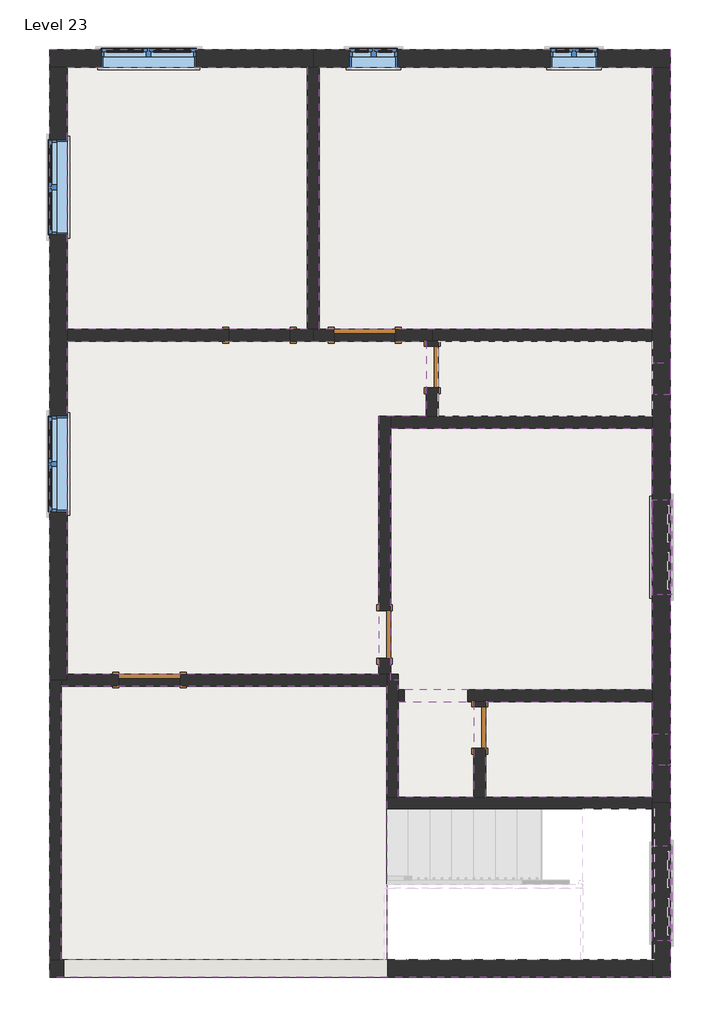
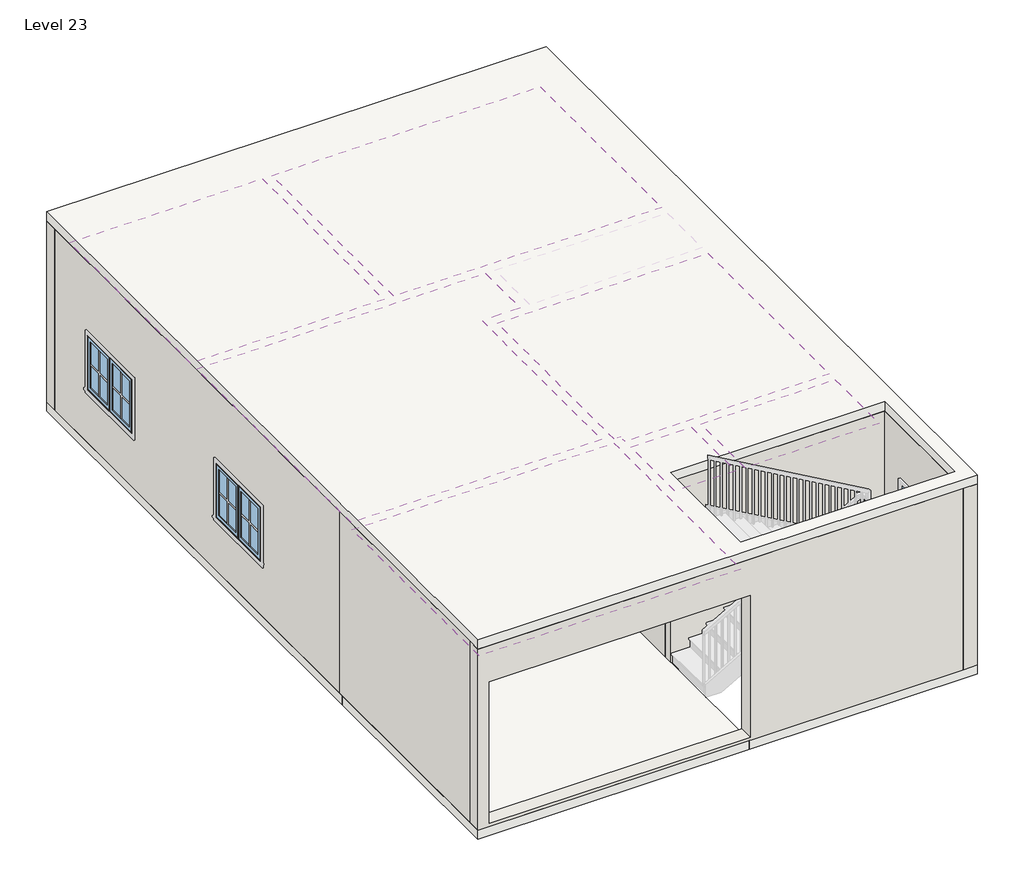
# One storey, part 1 of 2: 27 walls, 13 windows, 7 coverings, 6 doors, 3 slabs.
"""IFC4 building model written with IfcOpenShell, lengths in millimetres."""

from ifc_helpers import new_model, si_unit, frame, origin, place, context, project, spatial, polyline, outline, extrude, faceted_brep, transform, mapped, element, save
from components import door_2908be75, door_9ea4ff49, door_dc34e247, door_b804d09e, fixed_2_415b3208, window_casement_double_3_c417fced, window_casement_double_4_c19c33cb

model = new_model("IFC4")

# Units and contexts
model_context = context("Model", 3, world=origin())
ifc_project = project(units=[si_unit("LENGTHUNIT", "METRE", prefix="MILLI")], contexts=[model_context])

# Site, building, storey
site = spatial("IfcSite", under=ifc_project)
building = spatial("IfcBuilding", under=site)
storey = spatial("IfcBuildingStorey", under=building, Name="Level 23", Elevation=19202.4)

# Coverings
placement = place(None, origin())
element("IfcCovering", 1, ObjectType="2' x 4' ACT System", at=placement, inside=storey, context=model_context, shape_type="SweptSolid", body=[
    extrude(outline(polyline([(-5680.5154463, 2323.8455275), (-5680.5154463, 5678.2330275), (-2607.1154463, 5678.2330275), (-2607.1154463, 2323.8455275), (-5680.5154463, 2323.8455275)])), frame((0.0, 0.0, 21945.6), z_axis=(0.0, 0.0, 1.0), x_axis=(1.0, 0.0, 0.0)), (0.0, 0.0, 1.0), 57.15),
])
element("IfcCovering", 2, ObjectType="2' x 4' ACT System", at=placement, inside=storey, context=model_context, shape_type="SweptSolid", body=[
    extrude(outline(polyline([(-2454.7154463, 2323.8455275), (-2454.7154463, 5678.2330275), (1812.4845537, 5678.2330275), (1812.4845537, 2323.8455275), (-2454.7154463, 2323.8455275)])), frame((0.0, 0.0, 21945.6), z_axis=(0.0, 0.0, 1.0), x_axis=(1.0, 0.0, 0.0)), (0.0, 0.0, 1.0), 57.15),
])
element("IfcCovering", 3, ObjectType="2' x 4' ACT System", at=placement, inside=storey, context=model_context, shape_type="SweptSolid", body=[
    extrude(outline(polyline([(-5680.5154463, -2095.7544725), (-5680.5154463, 2171.4455275), (-1083.1154463, 2171.4455275), (-1083.1154463, 1206.2455275), (-1692.7154463, 1206.2455275), (-1692.7154463, -2095.7544725), (-5680.5154463, -2095.7544725)])), frame((0.0, 0.0, 21945.6), z_axis=(0.0, 0.0, 1.0), x_axis=(1.0, 0.0, 0.0)), (0.0, 0.0, 1.0), 57.15),
])
element("IfcCovering", 4, ObjectType="2' x 4' ACT System", at=placement, inside=storey, context=model_context, shape_type="SweptSolid", body=[
    extrude(outline(polyline([(1812.4845537, 1053.8455275), (1812.4845537, -2298.9544725), (-1438.7154463, -2298.9544725), (-1438.7154463, -2171.9544725), (-1540.3154463, -2171.9544725), (-1540.3154463, 1053.8455275), (1812.4845537, 1053.8455275)])), frame((0.0, 0.0, 21945.6), z_axis=(0.0, 0.0, 1.0), x_axis=(1.0, 0.0, 0.0)), (0.0, 0.0, 1.0), 57.15),
])
element("IfcCovering", 5, ObjectType="2' x 4' ACT System", at=placement, inside=storey, context=model_context, shape_type="SweptSolid", body=[
    extrude(outline(polyline([(1812.4845537, -2451.3544725), (1812.4845537, -3670.5544725), (-321.1154463, -3670.5544725), (-321.1154463, -2451.3544725), (1812.4845537, -2451.3544725)])), frame((0.0, 0.0, 21945.6), z_axis=(0.0, 0.0, 1.0), x_axis=(1.0, 0.0, 0.0)), (0.0, 0.0, 1.0), 57.15),
])
element("IfcCovering", 6, ObjectType="2' x 4' ACT System", at=placement, inside=storey, context=model_context, shape_type="SweptSolid", body=[
    extrude(outline(polyline([(-473.5154463, -2451.3544725), (-473.5154463, -3670.5544725), (-1438.7154463, -3670.5544725), (-1438.7154463, -2451.3544725), (-473.5154463, -2451.3544725)])), frame((0.0, 0.0, 21945.6), z_axis=(0.0, 0.0, 1.0), x_axis=(1.0, 0.0, 0.0)), (0.0, 0.0, 1.0), 57.15),
])
element("IfcCovering", 7, ObjectType="2' x 4' ACT System", at=placement, inside=storey, context=model_context, shape_type="SweptSolid", body=[
    extrude(outline(polyline([(-1591.1154463, -2248.1544725), (-1591.1154463, -5753.3544725), (-5756.7154463, -5753.3544725), (-5756.7154463, -2248.1544725), (-1591.1154463, -2248.1544725)])), frame((0.0, 0.0, 21945.6), z_axis=(0.0, 0.0, 1.0), x_axis=(1.0, 0.0, 0.0)), (0.0, 0.0, 1.0), 57.15),
])

# Doors
door_shape = door_2908be75(model_context)
element("IfcDoor", 8, ObjectType="Single-Flush : 1' 9\"", at=placement, inside=storey, context=model_context, shape_type="MappedRepresentation", body=[
    mapped(door_shape, transform((-397.3154463, -2781.5544725, 19202.4), x_axis=(0.0, 1.0, 0.0), y_axis=(-1.0, 0.0, 0.0), z_axis=(0.0, 0.0, 1.0))),
])
element("IfcDoor", 9, ObjectType="Single-Flush : 1' 9\"", at=placement, inside=storey, context=model_context, shape_type="MappedRepresentation", body=[
    mapped(door_shape, transform((-1006.9154463, 1841.2455275, 19202.4), x_axis=(0.0, 1.0, 0.0), y_axis=(-1.0, 0.0, 0.0), z_axis=(0.0, 0.0, 1.0))),
])
door_2_shape = door_9ea4ff49(model_context)
element("IfcDoor", 10, ObjectType="Single-Flush : 2'0\"", at=placement, inside=storey, context=model_context, shape_type="MappedRepresentation", body=[
    mapped(door_2_shape, transform((-1616.5154463, -1587.7544725, 19202.4), x_axis=(0.0, -1.0, 0.0), y_axis=(1.0, 0.0, 0.0), z_axis=(0.0, 0.0, 1.0))),
])
door_3_shape = door_dc34e247(model_context)
element("IfcDoor", 11, ObjectType="Single-Flush : 2'7\"", at=placement, inside=storey, context=model_context, shape_type="MappedRepresentation", body=[
    mapped(door_3_shape, transform((-4626.4154463, -2171.9544725, 19202.4), x_axis=(-1.0, 0.0, 0.0), y_axis=(0.0, -1.0, 0.0), z_axis=(0.0, 0.0, 1.0))),
])
element("IfcDoor", 12, ObjectType="Single-Flush : 2'7\"", at=placement, inside=storey, context=model_context, shape_type="MappedRepresentation", body=[
    mapped(door_3_shape, transform((-1870.5154463, 2247.6455275, 19202.4), x_axis=(-1.0, 0.0, 0.0), y_axis=(0.0, -1.0, 0.0), z_axis=(0.0, 0.0, 1.0))),
])
door_4_shape = door_b804d09e(model_context)
element("IfcDoor", 13, ObjectType="Single-Flush : 2'7\"", at=placement, inside=storey, context=model_context, shape_type="MappedRepresentation", body=[
    mapped(door_4_shape, transform((-3216.7154463, 2247.6455275, 19202.4), x_axis=(1.0, 0.0, 0.0), y_axis=(0.0, 1.0, 0.0), z_axis=(0.0, 0.0, 1.0))),
])

# Slabs
element("IfcSlab", 14, ObjectType="Generic - 6\"", at=placement, inside=storey, context=model_context, shape_type="SweptSolid", body=[
    extrude(outline(polyline([(-5909.1154463, -2248.1544725), (-5909.1154463, 5906.8330275), (2041.0845537, 5906.8330275), (2041.0845537, -5981.9544725), (-1591.1154463, -5981.9544725), (-1591.1154463, -5753.3544725), (1812.4845537, -5753.3544725), (1812.4845537, -3822.9544725), (-1591.1154463, -3822.9544725), (-1591.1154463, -2248.1544725), (-5756.7154463, -2248.1544725), (-5909.1154463, -2248.1544725)])), frame((0.0, 0.0, 19050.0), z_axis=(0.0, 0.0, 1.0), x_axis=(1.0, 0.0, 0.0)), (0.0, 0.0, 1.0), 152.4),
])
element("IfcSlab", 15, ObjectType="Generic - 6\"", at=placement, inside=storey, context=model_context, shape_type="SweptSolid", body=[
    extrude(outline(polyline([(-1591.1154463, -2248.1544725), (-1591.1154463, -5981.9544725), (-5909.1154463, -5981.9544725), (-5909.1154463, -2248.1544725), (-1591.1154463, -2248.1544725)])), frame((0.0, 0.0, 19050.0), z_axis=(0.0, 0.0, 1.0), x_axis=(1.0, 0.0, 0.0)), (0.0, 0.0, 1.0), 152.4),
])
element("IfcSlab", 16, ObjectType="Generic - 6\"", at=placement, inside=storey, context=model_context, shape_type="SweptSolid", body=[
    extrude(outline(polyline([(2041.0845537, 5906.8330275), (2041.0845537, -5981.9544725), (-5909.1154463, -5981.9544725), (-5909.1154463, 5906.8330275), (2041.0845537, 5906.8330275)]), holes=[polyline([(1812.4845537, -3822.9544725), (-1591.1154463, -3822.9544725), (-1591.1154463, -5753.3544725), (1812.4845537, -5753.3544725), (1812.4845537, -3822.9544725)])]), frame((0.0, 0.0, 22250.4), z_axis=(0.0, 0.0, 1.0), x_axis=(1.0, 0.0, 0.0)), (0.0, 0.0, 1.0), 152.4),
])

# Walls
element("IfcWall", 17, ObjectType="Generic - 6\"", at=placement, inside=storey, context=model_context, shape_type="Brep", body=[
    faceted_brep([(-5909.1154463, -2171.9544725, 19202.4), (-5909.1154463, -5753.3544725, 19202.4), (-5909.1154463, -5753.3544725, 22250.4), (-5909.1154463, -2171.9544725, 22250.4), (-5756.7154463, -2171.9544725, 19202.4), (-5756.7154463, -2171.9544725, 22250.4), (-5756.7154463, -2248.1544725, 22250.4), (-5756.7154463, -5753.3544725, 22250.4), (-5756.7154463, -5753.3544725, 19202.4), (-5756.7154463, -2248.1544725, 19202.4)], [[[0, 1, 2, 3]], [[4, 5, 6, 7, 8, 9]], [[1, 0, 4, 9, 8]], [[3, 2, 7, 6, 5]], [[0, 3, 5, 4]], [[2, 1, 8, 7]]]),
])
element("IfcWall", 18, ObjectType="Generic - 6\"", at=placement, inside=storey, context=model_context, shape_type="Brep", body=[
    faceted_brep([(1812.4845537, -3670.5544725, 19202.4), (-321.1154463, -3670.5544725, 19202.4), (-473.5154463, -3670.5544725, 19202.4), (-1438.7154463, -3670.5544725, 19202.4), (-1591.1154463, -3670.5544725, 19202.4), (-1591.1154463, -3670.5544725, 22250.4), (-1438.7154463, -3670.5544725, 22250.4), (-473.5154463, -3670.5544725, 22250.4), (-321.1154463, -3670.5544725, 22250.4), (1812.4845537, -3670.5544725, 22250.4), (1812.4845537, -3822.9544725, 19202.4), (1812.4845537, -3822.9544725, 22250.4), (-1591.1154463, -3822.9544725, 22250.4), (-1591.1154463, -3822.9544725, 19202.4), (1812.4845537, -3746.7544725, 19202.4), (1812.4845537, -3746.7544725, 22250.4)], [[[0, 1, 2, 3, 4, 5, 6, 7, 8, 9]], [[10, 11, 12, 13]], [[4, 3, 2, 1, 0, 14, 10, 13]], [[9, 8, 7, 6, 5, 12, 11, 15]], [[5, 4, 13, 12]], [[0, 9, 15, 11, 10, 14]]]),
])
element("IfcWall", 19, ObjectType="Generic - 6\"", at=placement, inside=storey, context=model_context, shape_type="Brep", body=[
    faceted_brep([(-1438.7154463, -3670.5544725, 19202.4), (-1438.7154463, -2451.3544725, 19202.4), (-1438.7154463, -2298.9544725, 19202.4), (-1438.7154463, -2095.7544725, 19202.4), (-1438.7154463, -2095.7544725, 22250.4), (-1438.7154463, -2298.9544725, 22250.4), (-1438.7154463, -2451.3544725, 22250.4), (-1438.7154463, -3670.5544725, 22250.4), (-1591.1154463, -3670.5544725, 19202.4), (-1591.1154463, -3670.5544725, 22250.4), (-1591.1154463, -2248.1544725, 22250.4), (-1591.1154463, -2171.9544725, 22250.4), (-1591.1154463, -2095.7544725, 22250.4), (-1591.1154463, -2095.7544725, 19202.4), (-1591.1154463, -2171.9544725, 19202.4), (-1591.1154463, -2248.1544725, 19202.4), (-1540.3154463, -2095.7544725, 19202.4), (-1540.3154463, -2095.7544725, 22250.4)], [[[0, 1, 2, 3, 4, 5, 6, 7]], [[8, 9, 10, 11, 12, 13, 14, 15]], [[3, 2, 1, 0, 8, 15, 14, 13, 16]], [[7, 6, 5, 4, 17, 12, 11, 10, 9]], [[0, 7, 9, 8]], [[4, 3, 16, 13, 12, 17]]]),
])
element("IfcWall", 20, ObjectType="Generic - 6\"", at=placement, inside=storey, context=model_context, shape_type="Brep", body=[
    faceted_brep([(-5020.1154463, -2095.7544725, 21336.0), (-5020.1154463, -2095.7544725, 19202.4), (-5680.5154463, -2095.7544725, 19202.4), (-5680.5154463, -2095.7544725, 22250.4), (-1692.7154463, -2095.7544725, 22250.4), (-1591.1154463, -2095.7544725, 22250.4), (-1591.1154463, -2095.7544725, 19202.4), (-1692.7154463, -2095.7544725, 19202.4), (-4232.7154463, -2095.7544725, 19202.4), (-4232.7154463, -2095.7544725, 21336.0), (-5756.7154463, -2248.1544725, 19202.4), (-5020.1154463, -2248.1544725, 19202.4), (-5020.1154463, -2248.1544725, 21336.0), (-4232.7154463, -2248.1544725, 21336.0), (-4232.7154463, -2248.1544725, 19202.4), (-1591.1154463, -2248.1544725, 19202.4), (-1591.1154463, -2248.1544725, 22250.4), (-5756.7154463, -2248.1544725, 22250.4), (-5756.7154463, -2171.9544725, 19202.4), (-5680.5154463, -2171.9544725, 19202.4), (-5680.5154463, -2171.9544725, 22250.4), (-5756.7154463, -2171.9544725, 22250.4)], [[[0, 1, 2, 3, 4, 5, 6, 7, 8, 9]], [[10, 11, 12, 13, 14, 15, 16, 17]], [[2, 1, 11, 10, 18, 19]], [[8, 7, 6, 15, 14]], [[5, 4, 3, 20, 21, 17, 16]], [[3, 2, 19, 20]], [[19, 18, 21, 20]], [[18, 10, 17, 21]], [[6, 5, 16, 15]], [[12, 11, 1, 0]], [[13, 12, 0, 9]], [[14, 13, 9, 8]]]),
])
element("IfcWall", 21, ObjectType="Generic - 6\"", at=placement, inside=storey, context=model_context, shape_type="Brep", body=[
    faceted_brep([(1812.4845537, -2451.3544725, 19202.4), (1812.4845537, -2451.3544725, 22250.4), (-321.1154463, -2451.3544725, 22250.4), (-473.5154463, -2451.3544725, 22250.4), (-1438.7154463, -2451.3544725, 22250.4), (-1438.7154463, -2451.3544725, 19202.4), (-1367.0206652, -2451.3544725, 19202.4), (-1367.0206652, -2451.3544725, 21640.8), (-547.4818767, -2451.3544725, 21640.8), (-547.4818767, -2451.3544725, 19202.4), (-473.5154463, -2451.3544725, 19202.4), (-321.1154463, -2451.3544725, 19202.4), (1812.4845537, -2298.9544725, 22250.4), (1812.4845537, -2298.9544725, 19202.4), (-547.4818767, -2298.9544725, 19202.4), (-547.4818767, -2298.9544725, 21640.8), (-1367.0206652, -2298.9544725, 21640.8), (-1367.0206652, -2298.9544725, 19202.4), (-1438.7154463, -2298.9544725, 19202.4), (-1438.7154463, -2298.9544725, 22250.4)], [[[0, 1, 2, 3, 4, 5, 6, 7, 8, 9, 10, 11]], [[12, 13, 14, 15, 16, 17, 18, 19]], [[5, 18, 17, 6]], [[13, 0, 11, 10, 9, 14]], [[4, 3, 2, 1, 12, 19]], [[1, 0, 13, 12]], [[5, 4, 19, 18]], [[7, 16, 15, 8]], [[16, 7, 6, 17]], [[8, 15, 14, 9]]]),
])
element("IfcWall", 22, ObjectType="Generic - 6\"", at=placement, inside=storey, context=model_context, shape_type="SweptSolid", body=[
    extrude(outline(polyline([(-2451.3544725, 19202.4), (-2514.8544725, 19202.4), (-2514.8544725, 21336.0), (-3048.2544725, 21336.0), (-3048.2544725, 19202.4), (-3670.5544725, 19202.4), (-3670.5544725, 22250.4), (-2451.3544725, 22250.4), (-2451.3544725, 19202.4)])), frame((-473.5154463, 0.0, 0.0), z_axis=(1.0, 0.0, 0.0), x_axis=(0.0, 1.0, 0.0)), (0.0, 0.0, 1.0), 152.4),
])
element("IfcWall", 23, ObjectType="Generic - 6\"", at=placement, inside=storey, context=model_context, shape_type="Brep", body=[
    faceted_brep([(-1540.3154463, -2095.7544725, 19202.4), (-1540.3154463, -1892.5544725, 19202.4), (-1540.3154463, -1892.5544725, 21336.0), (-1540.3154463, -1282.9544725, 21336.0), (-1540.3154463, -1282.9544725, 19202.4), (-1540.3154463, 1053.8455275, 19202.4), (-1540.3154463, 1206.2455275, 19202.4), (-1540.3154463, 1206.2455275, 22250.4), (-1540.3154463, 1053.8455275, 22250.4), (-1540.3154463, -2095.7544725, 22250.4), (-1692.7154463, -1892.5544725, 21336.0), (-1692.7154463, -1892.5544725, 19202.4), (-1692.7154463, -2095.7544725, 19202.4), (-1692.7154463, -2095.7544725, 22250.4), (-1692.7154463, 1206.2455275, 22250.4), (-1692.7154463, 1206.2455275, 19202.4), (-1692.7154463, -1282.9544725, 19202.4), (-1692.7154463, -1282.9544725, 21336.0), (-1591.1154463, -2095.7544725, 19202.4), (-1591.1154463, -2095.7544725, 22250.4)], [[[0, 1, 2, 3, 4, 5, 6, 7, 8, 9]], [[10, 11, 12, 13, 14, 15, 16, 17]], [[16, 15, 6, 5, 4]], [[12, 11, 1, 0, 18]], [[9, 8, 7, 14, 13, 19]], [[0, 9, 19, 13, 12, 18]], [[7, 6, 15, 14]], [[2, 1, 11, 10]], [[3, 2, 10, 17]], [[4, 3, 17, 16]]]),
])
element("IfcWall", 24, ObjectType="Generic - 6\"", at=placement, inside=storey, context=model_context, shape_type="Brep", body=[
    faceted_brep([(-1540.3154463, 1053.8455275, 19202.4), (1812.4845537, 1053.8455275, 19202.4), (1812.4845537, 1053.8455275, 22250.4), (-1540.3154463, 1053.8455275, 22250.4), (-1540.3154463, 1206.2455275, 19202.4), (-1540.3154463, 1206.2455275, 22250.4), (-1083.1154463, 1206.2455275, 22250.4), (-930.7154463, 1206.2455275, 22250.4), (1812.4845537, 1206.2455275, 22250.4), (1812.4845537, 1206.2455275, 19202.4), (-930.7154463, 1206.2455275, 19202.4), (-1083.1154463, 1206.2455275, 19202.4)], [[[0, 1, 2, 3]], [[4, 5, 6, 7, 8, 9, 10, 11]], [[1, 0, 4, 11, 10, 9]], [[3, 2, 8, 7, 6, 5]], [[0, 3, 5, 4]], [[2, 1, 9, 8]]]),
])
element("IfcWall", 25, ObjectType="Generic - 6\"", at=placement, inside=storey, context=model_context, shape_type="Brep", body=[
    faceted_brep([(-930.7154463, 2107.9455275, 21336.0), (-930.7154463, 2107.9455275, 19202.4), (-930.7154463, 2171.4455275, 19202.4), (-930.7154463, 2171.4455275, 22250.4), (-930.7154463, 1206.2455275, 22250.4), (-930.7154463, 1206.2455275, 19202.4), (-930.7154463, 1574.5455275, 19202.4), (-930.7154463, 1574.5455275, 21336.0), (-1083.1154463, 2171.4455275, 19202.4), (-1083.1154463, 2107.9455275, 19202.4), (-1083.1154463, 2107.9455275, 21336.0), (-1083.1154463, 1574.5455275, 21336.0), (-1083.1154463, 1574.5455275, 19202.4), (-1083.1154463, 1206.2455275, 19202.4), (-1083.1154463, 1206.2455275, 22250.4), (-1083.1154463, 2171.4455275, 22250.4), (-1006.9154463, 2171.4455275, 19202.4), (-1006.9154463, 2171.4455275, 22250.4)], [[[0, 1, 2, 3, 4, 5, 6, 7]], [[8, 9, 10, 11, 12, 13, 14, 15]], [[6, 5, 13, 12]], [[2, 1, 9, 8, 16]], [[4, 3, 17, 15, 14]], [[5, 4, 14, 13]], [[10, 9, 1, 0]], [[11, 10, 0, 7]], [[12, 11, 7, 6]], [[3, 2, 16, 8, 15, 17]]]),
])
element("IfcWall", 26, ObjectType="Generic - 6\"", at=placement, inside=storey, context=model_context, shape_type="Brep", body=[
    faceted_brep([(1812.4845537, 2323.8455275, 19202.4), (-1006.9154463, 2323.8455275, 19202.4), (-1006.9154463, 2323.8455275, 22250.4), (1812.4845537, 2323.8455275, 22250.4), (1812.4845537, 2171.4455275, 19202.4), (1812.4845537, 2171.4455275, 22250.4), (-930.7154463, 2171.4455275, 22250.4), (-1006.9154463, 2171.4455275, 22250.4), (-1006.9154463, 2171.4455275, 19202.4), (-930.7154463, 2171.4455275, 19202.4)], [[[0, 1, 2, 3]], [[4, 5, 6, 7, 8, 9]], [[1, 0, 4, 9, 8]], [[2, 1, 8, 7]], [[3, 2, 7, 6, 5]], [[0, 3, 5, 4]]]),
])
element("IfcWall", 27, ObjectType="Generic - 6\"", at=placement, inside=storey, context=model_context, shape_type="Brep", body=[
    faceted_brep([(-2607.1154463, 5678.2330275, 19202.4), (-2607.1154463, 2323.8455275, 19202.4), (-2607.1154463, 2323.8455275, 22250.4), (-2607.1154463, 5678.2330275, 22250.4), (-2454.7154463, 5678.2330275, 19202.4), (-2454.7154463, 5678.2330275, 22250.4), (-2454.7154463, 2323.8455275, 22250.4), (-2454.7154463, 2323.8455275, 19202.4), (-2530.9154463, 5678.2330275, 19202.4), (-2530.9154463, 2323.8455275, 19202.4), (-2530.9154463, 2323.8455275, 22250.4), (-2530.9154463, 5678.2330275, 22250.4)], [[[0, 1, 2, 3]], [[4, 5, 6, 7]], [[1, 0, 8, 4, 7, 9]], [[3, 2, 10, 6, 5, 11]], [[0, 3, 11, 5, 4, 8]], [[2, 1, 9, 7, 6, 10]]]),
])
element("IfcWall", 28, ObjectType="Generic - 6\"", at=placement, inside=storey, context=model_context, shape_type="Brep", body=[
    faceted_brep([(-2530.9154463, 2323.8455275, 19202.4), (-2607.1154463, 2323.8455275, 19202.4), (-2823.0154463, 2323.8455275, 19202.4), (-2823.0154463, 2323.8455275, 21336.0), (-3610.4154463, 2323.8455275, 21336.0), (-3610.4154463, 2323.8455275, 19202.4), (-5680.5154463, 2323.8455275, 19202.4), (-5680.5154463, 2323.8455275, 22250.4), (-2607.1154463, 2323.8455275, 22250.4), (-2530.9154463, 2323.8455275, 22250.4), (-2823.0154463, 2171.4455275, 21336.0), (-2823.0154463, 2171.4455275, 19202.4), (-2530.9154463, 2171.4455275, 19202.4), (-2530.9154463, 2171.4455275, 22250.4), (-5680.5154463, 2171.4455275, 22250.4), (-5680.5154463, 2171.4455275, 19202.4), (-3610.4154463, 2171.4455275, 19202.4), (-3610.4154463, 2171.4455275, 21336.0)], [[[0, 1, 2, 3, 4, 5, 6, 7, 8, 9]], [[10, 11, 12, 13, 14, 15, 16, 17]], [[16, 15, 6, 5]], [[12, 11, 2, 1, 0]], [[9, 8, 7, 14, 13]], [[0, 9, 13, 12]], [[7, 6, 15, 14]], [[5, 4, 17, 16]], [[4, 3, 10, 17]], [[3, 2, 11, 10]]]),
])
element("IfcWall", 29, ObjectType="Generic - 6\"", at=placement, inside=storey, context=model_context, shape_type="Brep", body=[
    faceted_brep([(-2264.2154463, 2323.8455275, 21336.0), (-2264.2154463, 2323.8455275, 19202.4), (-2454.7154463, 2323.8455275, 19202.4), (-2530.9154463, 2323.8455275, 19202.4), (-2530.9154463, 2323.8455275, 22250.4), (-2454.7154463, 2323.8455275, 22250.4), (-1006.9154463, 2323.8455275, 22250.4), (-1006.9154463, 2323.8455275, 19202.4), (-1476.8154463, 2323.8455275, 19202.4), (-1476.8154463, 2323.8455275, 21336.0), (-2530.9154463, 2171.4455275, 19202.4), (-2264.2154463, 2171.4455275, 19202.4), (-2264.2154463, 2171.4455275, 21336.0), (-1476.8154463, 2171.4455275, 21336.0), (-1476.8154463, 2171.4455275, 19202.4), (-1083.1154463, 2171.4455275, 19202.4), (-1006.9154463, 2171.4455275, 19202.4), (-1006.9154463, 2171.4455275, 22250.4), (-1083.1154463, 2171.4455275, 22250.4), (-2530.9154463, 2171.4455275, 22250.4)], [[[0, 1, 2, 3, 4, 5, 6, 7, 8, 9]], [[10, 11, 12, 13, 14, 15, 16, 17, 18, 19]], [[8, 7, 16, 15, 14]], [[3, 2, 1, 11, 10]], [[4, 3, 10, 19]], [[6, 5, 4, 19, 18, 17]], [[7, 6, 17, 16]], [[14, 13, 9, 8]], [[13, 12, 0, 9]], [[12, 11, 1, 0]]]),
])
element("IfcWall", 30, ObjectType="Generic - 6\"", at=placement, inside=storey, context=model_context, shape_type="SweptSolid", body=[
    extrude(outline(polyline([(-5680.5154463, -2095.7544725), (-1692.7154463, -2095.7544725), (-1692.7154463, -2171.9544725), (-1591.1154463, -2171.9544725), (-1591.1154463, -2248.1544725), (-5756.7154463, -2248.1544725), (-5756.7154463, -2171.9544725), (-5680.5154463, -2171.9544725), (-5680.5154463, -2095.7544725)])), frame((0.0, 0.0, 19202.4), z_axis=(0.0, 0.0, 1.0), x_axis=(1.0, 0.0, 0.0)), (0.0, 0.0, 1.0), 3048.0),
])
element("IfcWall", 31, ObjectType="Generic - 6\"", at=placement, inside=storey, context=model_context, shape_type="Brep", body=[
    faceted_brep([(-2607.1154463, 5678.2330275, 19202.4), (-2607.1154463, 2323.8455275, 19202.4), (-2607.1154463, 2323.8455275, 22250.4), (-2607.1154463, 5678.2330275, 22250.4), (-2454.7154463, 5678.2330275, 19202.4), (-2454.7154463, 5678.2330275, 22250.4), (-2454.7154463, 2323.8455275, 22250.4), (-2454.7154463, 2323.8455275, 19202.4), (-2530.9154463, 5678.2330275, 19202.4), (-2530.9154463, 2323.8455275, 19202.4), (-2530.9154463, 2323.8455275, 22250.4), (-2530.9154463, 5678.2330275, 22250.4)], [[[0, 1, 2, 3]], [[4, 5, 6, 7]], [[1, 0, 8, 4, 7, 9]], [[3, 2, 10, 6, 5, 11]], [[0, 3, 11, 5, 4, 8]], [[2, 1, 9, 7, 6, 10]]]),
])
element("IfcWall", 32, ObjectType="Generic - 6\"", at=placement, inside=storey, context=model_context, shape_type="Brep", body=[
    faceted_brep([(-2530.9154463, 2323.8455275, 19202.4), (-2607.1154463, 2323.8455275, 19202.4), (-5680.5154463, 2323.8455275, 19202.4), (-5680.5154463, 2323.8455275, 22250.4), (-2607.1154463, 2323.8455275, 22250.4), (-2530.9154463, 2323.8455275, 22250.4), (-2530.9154463, 2171.4455275, 19202.4), (-2530.9154463, 2171.4455275, 22250.4), (-5680.5154463, 2171.4455275, 22250.4), (-5680.5154463, 2171.4455275, 19202.4)], [[[0, 1, 2, 3, 4, 5]], [[6, 7, 8, 9]], [[2, 1, 0, 6, 9]], [[5, 4, 3, 8, 7]], [[0, 5, 7, 6]], [[3, 2, 9, 8]]]),
])
element("IfcWall", 33, ObjectType="Generic - 6\"", at=placement, inside=storey, context=model_context, shape_type="Brep", body=[
    faceted_brep([(-1006.9154463, 2323.8455275, 19202.4), (-2454.7154463, 2323.8455275, 19202.4), (-2530.9154463, 2323.8455275, 19202.4), (-2530.9154463, 2323.8455275, 22250.4), (-2454.7154463, 2323.8455275, 22250.4), (-1006.9154463, 2323.8455275, 22250.4), (-1006.9154463, 2171.4455275, 19202.4), (-1006.9154463, 2171.4455275, 22250.4), (-1083.1154463, 2171.4455275, 22250.4), (-2530.9154463, 2171.4455275, 22250.4), (-2530.9154463, 2171.4455275, 19202.4), (-1083.1154463, 2171.4455275, 19202.4)], [[[0, 1, 2, 3, 4, 5]], [[6, 7, 8, 9, 10, 11]], [[2, 1, 0, 6, 11, 10]], [[3, 2, 10, 9]], [[5, 4, 3, 9, 8, 7]], [[0, 5, 7, 6]]]),
])
element("IfcWall", 34, ObjectType="Generic - 9\"", at=placement, inside=storey, context=model_context, shape_type="Brep", body=[
    faceted_brep([(-5909.1154463, 5678.2330275, 19202.4), (-5680.5154463, 5678.2330275, 19202.4), (-2607.1154463, 5678.2330275, 19202.4), (-2530.9154463, 5678.2330275, 19202.4), (-2530.9154463, 5678.2330275, 22250.4), (-2607.1154463, 5678.2330275, 22250.4), (-5680.5154463, 5678.2330275, 22250.4), (-5909.1154463, 5678.2330275, 22250.4), (-4029.5154463, 5678.2330275, 21031.2), (-4029.5154463, 5678.2330275, 20116.8), (-5248.7154463, 5678.2330275, 20116.8), (-5248.7154463, 5678.2330275, 21031.2), (-5909.1154463, 5906.8330275, 19202.4), (-5909.1154463, 5906.8330275, 22250.4), (-2530.9154463, 5906.8330275, 22250.4), (-2530.9154463, 5906.8330275, 19202.4), (-4029.5154463, 5906.8330275, 21031.2), (-5248.7154463, 5906.8330275, 21031.2), (-5248.7154463, 5906.8330275, 20116.8), (-4029.5154463, 5906.8330275, 20116.8)], [[[0, 1, 2, 3, 4, 5, 6, 7], [8, 9, 10, 11]], [[12, 13, 14, 15], [16, 17, 18, 19]], [[3, 2, 1, 0, 12, 15]], [[4, 3, 15, 14]], [[7, 6, 5, 4, 14, 13]], [[0, 7, 13, 12]], [[9, 8, 16, 19]], [[10, 9, 19, 18]], [[11, 10, 18, 17]], [[8, 11, 17, 16]]]),
])
element("IfcWall", 35, ObjectType="Generic - 9\"", at=placement, inside=storey, context=model_context, shape_type="Brep", body=[
    faceted_brep([(1812.4845537, 5678.2330275, 19202.4), (1812.4845537, 2323.8455275, 19202.4), (1812.4845537, 2171.4455275, 19202.4), (1812.4845537, 1206.2455275, 19202.4), (1812.4845537, 1053.8455275, 19202.4), (1812.4845537, -2298.9544725, 19202.4), (1812.4845537, -2451.3544725, 19202.4), (1812.4845537, -3670.5544725, 19202.4), (1812.4845537, -3746.7544725, 19202.4), (1812.4845537, -3746.7544725, 22250.4), (1812.4845537, -3670.5544725, 22250.4), (1812.4845537, -2451.3544725, 22250.4), (1812.4845537, -2298.9544725, 22250.4), (1812.4845537, 1053.8455275, 22250.4), (1812.4845537, 1206.2455275, 22250.4), (1812.4845537, 2171.4455275, 22250.4), (1812.4845537, 2323.8455275, 22250.4), (1812.4845537, 5678.2330275, 22250.4), (1812.4845537, -1079.7544725, 21336.0), (1812.4845537, -1079.7544725, 20421.6), (1812.4845537, 139.4455275, 20421.6), (1812.4845537, 139.4455275, 21336.0), (1812.4845537, -3264.1544725, 21640.8), (1812.4845537, -3264.1544725, 21031.2), (1812.4845537, -2857.7544725, 21031.2), (1812.4845537, -2857.7544725, 21640.8), (1812.4845537, 1892.0455275, 21640.8), (1812.4845537, 1485.6455275, 21640.8), (1812.4845537, 1485.6455275, 21031.2), (1812.4845537, 1892.0455275, 21031.2), (2041.0845537, 5678.2330275, 19202.4), (2041.0845537, 5678.2330275, 22250.4), (2041.0845537, -3746.7544725, 22250.4), (2041.0845537, -3746.7544725, 19202.4), (2041.0845537, -1079.7544725, 21336.0), (2041.0845537, 139.4455275, 21336.0), (2041.0845537, 139.4455275, 20421.6), (2041.0845537, -1079.7544725, 20421.6), (2041.0845537, -3264.1544725, 21640.8), (2041.0845537, -2857.7544725, 21640.8), (2041.0845537, -2857.7544725, 21031.2), (2041.0845537, -3264.1544725, 21031.2), (2041.0845537, 1892.0455275, 21640.8), (2041.0845537, 1892.0455275, 21031.2), (2041.0845537, 1485.6455275, 21031.2), (2041.0845537, 1485.6455275, 21640.8)], [[[0, 1, 2, 3, 4, 5, 6, 7, 8, 9, 10, 11, 12, 13, 14, 15, 16, 17], [18, 19, 20, 21], [22, 23, 24, 25], [26, 27, 28, 29]], [[30, 31, 32, 33], [34, 35, 36, 37], [38, 39, 40, 41], [42, 43, 44, 45]], [[8, 7, 6, 5, 4, 3, 2, 1, 0, 30, 33]], [[9, 8, 33, 32]], [[17, 16, 15, 14, 13, 12, 11, 10, 9, 32, 31]], [[0, 17, 31, 30]], [[19, 18, 34, 37]], [[20, 19, 37, 36]], [[21, 20, 36, 35]], [[18, 21, 35, 34]], [[23, 22, 38, 41]], [[24, 23, 41, 40]], [[25, 24, 40, 39]], [[22, 25, 39, 38]], [[43, 42, 26, 29]], [[44, 43, 29, 28]], [[45, 44, 28, 27]], [[42, 45, 27, 26]]]),
])
element("IfcWall", 36, ObjectType="Generic - 9\"", at=placement, inside=storey, context=model_context, shape_type="Brep", body=[
    faceted_brep([(1812.4845537, -5753.3544725, 19202.4), (-5756.7154463, -5753.3544725, 19202.4), (-5909.1154463, -5753.3544725, 19202.4), (-5909.1154463, -5753.3544725, 22250.4), (-5756.7154463, -5753.3544725, 22250.4), (1812.4845537, -5753.3544725, 22250.4), (-1576.8982041, -5753.3544725, 21640.8), (-5729.1673724, -5753.3544725, 21640.8), (-5729.1673724, -5753.3544725, 19253.2), (-1576.8982041, -5753.3544725, 19253.2), (-5909.1154463, -5981.9544725, 19202.4), (1812.4845537, -5981.9544725, 19202.4), (1812.4845537, -5981.9544725, 22250.4), (-5909.1154463, -5981.9544725, 22250.4), (-5729.1673724, -5981.9544725, 21640.8), (-1576.8982041, -5981.9544725, 21640.8), (-1576.8982041, -5981.9544725, 19253.2), (-5729.1673724, -5981.9544725, 19253.2)], [[[0, 1, 2, 3, 4, 5], [6, 7, 8, 9]], [[10, 11, 12, 13], [14, 15, 16, 17]], [[2, 1, 0, 11, 10]], [[5, 4, 3, 13, 12]], [[0, 5, 12, 11]], [[6, 15, 14, 7]], [[8, 17, 16, 9]], [[15, 6, 9, 16]], [[7, 14, 17, 8]], [[3, 2, 10, 13]]]),
])
element("IfcWall", 37, ObjectType="Generic - 9\"", at=placement, inside=storey, context=model_context, shape_type="Brep", body=[
    faceted_brep([(-5909.1154463, 5678.2330275, 19202.4), (-5909.1154463, -2171.9544725, 19202.4), (-5909.1154463, -2171.9544725, 22250.4), (-5909.1154463, 5678.2330275, 22250.4), (-5909.1154463, 4751.1330275, 21031.2), (-5909.1154463, 3531.9330275, 21031.2), (-5909.1154463, 3531.9330275, 20116.8), (-5909.1154463, 4751.1330275, 20116.8), (-5909.1154463, 1206.2455275, 21031.2), (-5909.1154463, -12.9544725, 21031.2), (-5909.1154463, -12.9544725, 20116.8), (-5909.1154463, 1206.2455275, 20116.8), (-5680.5154463, 5678.2330275, 19202.4), (-5680.5154463, 5678.2330275, 22250.4), (-5680.5154463, 2323.8455275, 22250.4), (-5680.5154463, 2171.4455275, 22250.4), (-5680.5154463, -2095.7544725, 22250.4), (-5680.5154463, -2171.9544725, 22250.4), (-5680.5154463, -2171.9544725, 19202.4), (-5680.5154463, -2095.7544725, 19202.4), (-5680.5154463, 2171.4455275, 19202.4), (-5680.5154463, 2323.8455275, 19202.4), (-5680.5154463, 4751.1330275, 21031.2), (-5680.5154463, 4751.1330275, 20116.8), (-5680.5154463, 3531.9330275, 20116.8), (-5680.5154463, 3531.9330275, 21031.2), (-5680.5154463, 1206.2455275, 21031.2), (-5680.5154463, 1206.2455275, 20116.8), (-5680.5154463, -12.9544725, 20116.8), (-5680.5154463, -12.9544725, 21031.2), (-5756.7154463, -2171.9544725, 19202.4), (-5756.7154463, -2171.9544725, 22250.4)], [[[0, 1, 2, 3], [4, 5, 6, 7], [8, 9, 10, 11]], [[12, 13, 14, 15, 16, 17, 18, 19, 20, 21], [22, 23, 24, 25], [26, 27, 28, 29]], [[1, 0, 12, 21, 20, 19, 18, 30]], [[2, 1, 30, 18, 17, 31]], [[3, 2, 31, 17, 16, 15, 14, 13]], [[0, 3, 13, 12]], [[23, 22, 4, 7]], [[24, 23, 7, 6]], [[25, 24, 6, 5]], [[22, 25, 5, 4]], [[27, 26, 8, 11]], [[28, 27, 11, 10]], [[29, 28, 10, 9]], [[26, 29, 9, 8]]]),
])
element("IfcWall", 38, ObjectType="Generic - 9\"", at=placement, inside=storey, context=model_context, shape_type="Brep", body=[
    faceted_brep([(-2530.9154463, 5678.2330275, 19202.4), (-2454.7154463, 5678.2330275, 19202.4), (1812.4845537, 5678.2330275, 19202.4), (2041.0845537, 5678.2330275, 19202.4), (2041.0845537, 5678.2330275, 22250.4), (1812.4845537, 5678.2330275, 22250.4), (-2454.7154463, 5678.2330275, 22250.4), (-2530.9154463, 5678.2330275, 22250.4), (-1451.4154463, 5678.2330275, 21031.2), (-1451.4154463, 5678.2330275, 20116.8), (-2061.0154463, 5678.2330275, 20116.8), (-2061.0154463, 5678.2330275, 21031.2), (1113.9845537, 5678.2330275, 21031.2), (1113.9845537, 5678.2330275, 20116.8), (504.3845537, 5678.2330275, 20116.8), (504.3845537, 5678.2330275, 21031.2), (-2530.9154463, 5906.8330275, 19202.4), (-2530.9154463, 5906.8330275, 22250.4), (2041.0845537, 5906.8330275, 22250.4), (2041.0845537, 5906.8330275, 19202.4), (-1451.4154463, 5906.8330275, 21031.2), (-2061.0154463, 5906.8330275, 21031.2), (-2061.0154463, 5906.8330275, 20116.8), (-1451.4154463, 5906.8330275, 20116.8), (1113.9845537, 5906.8330275, 21031.2), (504.3845537, 5906.8330275, 21031.2), (504.3845537, 5906.8330275, 20116.8), (1113.9845537, 5906.8330275, 20116.8)], [[[0, 1, 2, 3, 4, 5, 6, 7], [8, 9, 10, 11], [12, 13, 14, 15]], [[16, 17, 18, 19], [20, 21, 22, 23], [24, 25, 26, 27]], [[3, 2, 1, 0, 16, 19]], [[7, 6, 5, 4, 18, 17]], [[0, 7, 17, 16]], [[4, 3, 19, 18]], [[8, 11, 21, 20]], [[11, 10, 22, 21]], [[10, 9, 23, 22]], [[9, 8, 20, 23]], [[12, 15, 25, 24]], [[15, 14, 26, 25]], [[14, 13, 27, 26]], [[13, 12, 24, 27]]]),
])
element("IfcWall", 39, ObjectType="Generic - 9\"", at=placement, inside=storey, context=model_context, shape_type="Brep", body=[
    faceted_brep([(1812.4845537, -3746.7544725, 19202.4), (1812.4845537, -3822.9544725, 19202.4), (1812.4845537, -5753.3544725, 19202.4), (1812.4845537, -5981.9544725, 19202.4), (1812.4845537, -5981.9544725, 22250.4), (1812.4845537, -5753.3544725, 22250.4), (1812.4845537, -3822.9544725, 22250.4), (1812.4845537, -3746.7544725, 22250.4), (1812.4845537, -5512.0544725, 21336.0), (1812.4845537, -5512.0544725, 20421.6), (1812.4845537, -4292.8544725, 20421.6), (1812.4845537, -4292.8544725, 21336.0), (2041.0845537, -3746.7544725, 19202.4), (2041.0845537, -3746.7544725, 22250.4), (2041.0845537, -5981.9544725, 22250.4), (2041.0845537, -5981.9544725, 19202.4), (2041.0845537, -5512.0544725, 21336.0), (2041.0845537, -4292.8544725, 21336.0), (2041.0845537, -4292.8544725, 20421.6), (2041.0845537, -5512.0544725, 20421.6)], [[[0, 1, 2, 3, 4, 5, 6, 7], [8, 9, 10, 11]], [[12, 13, 14, 15], [16, 17, 18, 19]], [[3, 2, 1, 0, 12, 15]], [[7, 6, 5, 4, 14, 13]], [[0, 7, 13, 12]], [[4, 3, 15, 14]], [[8, 11, 17, 16]], [[11, 10, 18, 17]], [[10, 9, 19, 18]], [[9, 8, 16, 19]]]),
])
element("IfcWall", 40, ObjectType="Generic - 9\"", at=placement, inside=storey, context=model_context, shape_type="SweptSolid", body=[
    extrude(outline(polyline([(19202.4, -5680.5154463), (19202.4, -2607.1154463), (22250.4, -2607.1154463), (22250.4, -5680.5154463), (19202.4, -5680.5154463)]), holes=[polyline([(21031.2, -4029.5154463), (20116.8, -4029.5154463), (20116.8, -5248.7154463), (21031.2, -5248.7154463), (21031.2, -4029.5154463)])]), frame((0.0, 5678.2330275, 0.0), z_axis=(0.0, 1.0, 0.0), x_axis=(0.0, 0.0, 1.0)), (0.0, 0.0, 1.0), 228.6),
])
element("IfcWall", 41, ObjectType="Generic - 9\"", at=placement, inside=storey, context=model_context, shape_type="Brep", body=[
    faceted_brep([(1812.4845537, -5753.3544725, 19202.4), (-5756.7154463, -5753.3544725, 19202.4), (-5909.1154463, -5753.3544725, 19202.4), (-5909.1154463, -5753.3544725, 22250.4), (-5756.7154463, -5753.3544725, 22250.4), (1812.4845537, -5753.3544725, 22250.4), (-1576.8982041, -5753.3544725, 21640.8), (-5729.1673724, -5753.3544725, 21640.8), (-5729.1673724, -5753.3544725, 19253.2), (-1576.8982041, -5753.3544725, 19253.2), (-5909.1154463, -5981.9544725, 19202.4), (1812.4845537, -5981.9544725, 19202.4), (1812.4845537, -5981.9544725, 22250.4), (-5909.1154463, -5981.9544725, 22250.4), (-5729.1673724, -5981.9544725, 21640.8), (-1576.8982041, -5981.9544725, 21640.8), (-1576.8982041, -5981.9544725, 19253.2), (-5729.1673724, -5981.9544725, 19253.2)], [[[0, 1, 2, 3, 4, 5], [6, 7, 8, 9]], [[10, 11, 12, 13], [14, 15, 16, 17]], [[2, 1, 0, 11, 10]], [[5, 4, 3, 13, 12]], [[6, 15, 14, 7]], [[8, 17, 16, 9]], [[15, 6, 9, 16]], [[7, 14, 17, 8]], [[3, 2, 10, 13]], [[0, 5, 12, 11]]]),
])
element("IfcWall", 42, ObjectType="Generic - 9\"", at=placement, inside=storey, context=model_context, shape_type="SweptSolid", body=[
    extrude(outline(polyline([(19202.4, -2454.7154463), (19202.4, 1812.4845537), (22250.4, 1812.4845537), (22250.4, -2454.7154463), (19202.4, -2454.7154463)]), holes=[polyline([(21031.2, -1451.4154463), (20116.8, -1451.4154463), (20116.8, -2061.0154463), (21031.2, -2061.0154463), (21031.2, -1451.4154463)]), polyline([(21031.2, 1113.9845537), (20116.8, 1113.9845537), (20116.8, 504.3845537), (21031.2, 504.3845537), (21031.2, 1113.9845537)])]), frame((0.0, 5678.2330275, 0.0), z_axis=(0.0, 1.0, 0.0), x_axis=(0.0, 0.0, 1.0)), (0.0, 0.0, 1.0), 228.6),
])
element("IfcWall", 43, ObjectType="Generic - 9\"", at=placement, inside=storey, context=model_context, shape_type="SweptSolid", body=[
    extrude(outline(polyline([(-3822.9544725, 19202.4), (-5753.3544725, 19202.4), (-5753.3544725, 22250.4), (-3822.9544725, 22250.4), (-3822.9544725, 19202.4)]), holes=[polyline([(-5512.0544725, 21336.0), (-5512.0544725, 20421.6), (-4292.8544725, 20421.6), (-4292.8544725, 21336.0), (-5512.0544725, 21336.0)])]), frame((1812.4845537, 0.0, 0.0), z_axis=(1.0, 0.0, 0.0), x_axis=(0.0, 1.0, 0.0)), (0.0, 0.0, 1.0), 228.6),
])

# Windows
fixed_2_shape = fixed_2_415b3208(model_context)
element("IfcWindow", 44, ObjectType="Fixed : 2'", at=placement, inside=storey, context=model_context, shape_type="MappedRepresentation", body=[
    mapped(fixed_2_shape, transform((1926.7845537, -3099.0544725, 20726.4), x_axis=(0.0, -1.0, 0.0), y_axis=(1.0, 0.0, 0.0), z_axis=(0.0, 0.0, 1.0))),
])
element("IfcWindow", 45, ObjectType="Fixed : 2'", at=placement, inside=storey, context=model_context, shape_type="MappedRepresentation", body=[
    mapped(fixed_2_shape, transform((1926.7845537, 1726.9455275, 20726.4), x_axis=(0.0, 1.0, 0.0), y_axis=(-1.0, 0.0, 0.0), z_axis=(0.0, 0.0, 1.0))),
])
window_casement_double_3_shape = window_casement_double_3_c417fced(model_context)
element("IfcWindow", 46, ObjectType="Window-Casement-Double : 3'", at=placement, inside=storey, context=model_context, shape_type="MappedRepresentation", body=[
    mapped(window_casement_double_3_shape, transform((-1756.2154463, 5792.5330275, 19202.4), x_axis=(1.0, 0.0, 0.0), y_axis=(0.0, 1.0, 0.0), z_axis=(0.0, 0.0, 1.0))),
])
element("IfcWindow", 47, ObjectType="Window-Casement-Double : 3'", at=placement, inside=storey, context=model_context, shape_type="MappedRepresentation", body=[
    mapped(window_casement_double_3_shape, transform((809.1845537, 5792.5330275, 19202.4), x_axis=(1.0, 0.0, 0.0), y_axis=(0.0, 1.0, 0.0), z_axis=(0.0, 0.0, 1.0))),
])
element("IfcWindow", 48, ObjectType="Window-Casement-Double : 3'", at=placement, inside=storey, context=model_context, shape_type="MappedRepresentation", body=[
    mapped(window_casement_double_3_shape, transform((-1756.2154463, 5792.5330275, 19202.4), x_axis=(1.0, 0.0, 0.0), y_axis=(0.0, 1.0, 0.0), z_axis=(0.0, 0.0, 1.0))),
])
element("IfcWindow", 49, ObjectType="Window-Casement-Double : 3'", at=placement, inside=storey, context=model_context, shape_type="MappedRepresentation", body=[
    mapped(window_casement_double_3_shape, transform((809.1845537, 5792.5330275, 19202.4), x_axis=(1.0, 0.0, 0.0), y_axis=(0.0, 1.0, 0.0), z_axis=(0.0, 0.0, 1.0))),
])
window_casement_double_4_shape = window_casement_double_4_c19c33cb(model_context)
element("IfcWindow", 50, ObjectType="Window-Casement-Double : 4'", at=placement, inside=storey, context=model_context, shape_type="MappedRepresentation", body=[
    mapped(window_casement_double_4_shape, transform((-4639.1154463, 5792.5330275, 19202.4), x_axis=(1.0, 0.0, 0.0), y_axis=(0.0, 1.0, 0.0), z_axis=(0.0, 0.0, 1.0))),
])
element("IfcWindow", 51, ObjectType="Window-Casement-Double : 4'", at=placement, inside=storey, context=model_context, shape_type="MappedRepresentation", body=[
    mapped(window_casement_double_4_shape, transform((-5794.8154463, 4141.5330275, 19202.4), x_axis=(0.0, 1.0, 0.0), y_axis=(-1.0, 0.0, 0.0), z_axis=(0.0, 0.0, 1.0))),
])
element("IfcWindow", 52, ObjectType="Window-Casement-Double : 4'", at=placement, inside=storey, context=model_context, shape_type="MappedRepresentation", body=[
    mapped(window_casement_double_4_shape, transform((-5794.8154463, 596.6455275, 19202.4), x_axis=(0.0, 1.0, 0.0), y_axis=(-1.0, 0.0, 0.0), z_axis=(0.0, 0.0, 1.0))),
])
element("IfcWindow", 53, ObjectType="Window-Casement-Double : 4'", at=placement, inside=storey, context=model_context, shape_type="MappedRepresentation", body=[
    mapped(window_casement_double_4_shape, transform((1926.7845537, -470.1544725, 19507.2), x_axis=(0.0, -1.0, 0.0), y_axis=(1.0, 0.0, 0.0), z_axis=(0.0, 0.0, 1.0))),
])
element("IfcWindow", 54, ObjectType="Window-Casement-Double : 4'", at=placement, inside=storey, context=model_context, shape_type="MappedRepresentation", body=[
    mapped(window_casement_double_4_shape, transform((1926.7845537, -4902.4544725, 19507.2), x_axis=(0.0, -1.0, 0.0), y_axis=(1.0, 0.0, 0.0), z_axis=(0.0, 0.0, 1.0))),
])
element("IfcWindow", 55, ObjectType="Window-Casement-Double : 4'", at=placement, inside=storey, context=model_context, shape_type="MappedRepresentation", body=[
    mapped(window_casement_double_4_shape, transform((-4639.1154463, 5792.5330275, 19202.4), x_axis=(1.0, 0.0, 0.0), y_axis=(0.0, 1.0, 0.0), z_axis=(0.0, 0.0, 1.0))),
])
element("IfcWindow", 56, ObjectType="Window-Casement-Double : 4'", at=placement, inside=storey, context=model_context, shape_type="MappedRepresentation", body=[
    mapped(window_casement_double_4_shape, transform((1926.7845537, -4902.4544725, 19507.2), x_axis=(0.0, -1.0, 0.0), y_axis=(1.0, 0.0, 0.0), z_axis=(0.0, 0.0, 1.0))),
])

save(model, "model.ifc")

# Revit data of these elements
# Type "2' x 4' ACT System"
#   Assembly Code = "C3030210"
#   built-in parameter 1002203 = 1 (stored number, unit not read)
#   built-in parameter 1002202 = 1 (stored number, unit not read)
#   Layers, outside or top first: 0' - 1 5/8" "Default" (function 1); 0' - 0 5/8" "Acoustic Ceiling Tile 24 x 48" (function 5)
# Type "Single-Flush : 1' 9\""
#   Type Mark = "10"
#   Construction Type Id = "MDOOR"
#   Assembly Code = "C1020"
#   Analytic Construction = "Metal"
#   Thickness = 0' - 2"
#   Heat Transfer Coefficient (U) = 0.651978 BTU/(h·ft²·°F)
#   Height = 7' - 0"
#   Trim Projection Ext = 0' - 1"
#   Trim Projection Int = 0' - 1"
#   Trim Width = 0' - 3"
#   Width = 1' - 9"
#   Define Thermal Properties by = 1
#   Door Material = Door - Panel
#   Frame Material = Door - Frame
#   Visual Light Transmittance = 0
#   Solar Heat Gain Coefficient = 0
#   Function = (empty or 0)
#   Wall Closure = (empty or 0)
# Type "Single-Flush : 2'0\""
#   Type Mark = "9"
#   Construction Type Id = "MDOOR"
#   Assembly Code = "C1020"
#   Analytic Construction = "Metal"
#   Thickness = 0' - 2"
#   Heat Transfer Coefficient (U) = 0.651978 BTU/(h·ft²·°F)
#   Height = 7' - 0"
#   Trim Projection Ext = 0' - 1"
#   Trim Projection Int = 0' - 1"
#   Trim Width = 0' - 3"
#   Width = 2' - 0"
#   Define Thermal Properties by = 1
#   Door Material = Door - Panel
#   Frame Material = Door - Frame
#   Visual Light Transmittance = 0
#   Solar Heat Gain Coefficient = 0
#   Function = (empty or 0)
#   Wall Closure = (empty or 0)
# Type "Single-Flush : 2'7\""
#   Type Mark = "8"
#   Construction Type Id = "MDOOR"
#   Assembly Code = "C1020"
#   Analytic Construction = "Metal"
#   Thickness = 0' - 2"
#   Heat Transfer Coefficient (U) = 0.651978 BTU/(h·ft²·°F)
#   Height = 7' - 0"
#   Trim Projection Ext = 0' - 1"
#   Trim Projection Int = 0' - 1"
#   Trim Width = 0' - 3"
#   Width = 2' - 7"
#   Define Thermal Properties by = 1
#   Door Material = Door - Panel
#   Frame Material = Door - Frame
#   Visual Light Transmittance = 0
#   Solar Heat Gain Coefficient = 0
#   Function = (empty or 0)
#   Wall Closure = (empty or 0)
# Type "Generic - 6\""
#   Assembly Code = "B1010"
#   Function = 0
#   Layers, outside or top first: 0' - 6" no material (function 1)
# Type "Generic - 6\""
#   Assembly Code = "B2010"
#   Layers, outside or top first: 0' - 6" no material (function 1)
# Type "Generic - 9\""
#   Assembly Code = "B2010"
#   Layers, outside or top first: 0' - 9" no material (function 1)
# Type "Fixed : 2'"
#   Type Mark = "20"
#   Construction Type Id = "GSP4R"
#   Assembly Code = "B2020100"
#   Analytic Construction = "1/8 in Pilkington single glazing"
#   Visual Light Transmittance = 0.9
#   Solar Heat Gain Coefficient = 0.78
#   Heat Transfer Coefficient (U) = 0.6496 BTU/(h·ft²·°F)
#   Height = 2' - 0"
#   Default Sill Height = 1' - 0"
#   Width = 1' - 4"
#   Window Inset = 0' - 0 3/4"
#   Define Thermal Properties by = 1
#   Glass Pane Material = Glass
#   Sash Material = Sash
#   Wall Closure = (empty or 0)
# Type "Window-Casement-Double : 3'"
#   Type Mark = "19"
#   Fire Rating = "0.5h"
#   Assembly Code = "B2020100"
#   Analytic Construction = "Double glazing - domestic"
#   Frame Extension [instance default] = 0' - 0 1/4"
#   Window Inset [instance default] = 0' - 0"
#   Wall Thickness [instance default] = 0' - 6"
#   Interior Wall Closure [instance default] = 0' - 2 1/4"
#   Half Width = 1' - 0"
#   Visual Light Transmittance = 0.81
#   Thermal Resistance (R) = 1.8146 (h·ft²·°F)/BTU
#   Solar Heat Gain Coefficient = 0.76
#   Rough Width = 2' - 0 1/2"
#   Rough Height = 3' - 0 1/2"
#   Height = 3' - 0"
#   Heat Transfer Coefficient (U) = 0.5511 BTU/(h·ft²·°F)
#   Exterior Wall Closure [instance default] = 0' - 1 1/4"
#   Extension Jamb [instance default] = 0' - 2 1/4"
#   Default Sill Height = 3' - 0"
#   Width = 2' - 0"
#   Muntin Visibility = yes
#   Interior Trim Visibility [instance default] = yes
#   Exterior Trim Visibility [instance default] = yes
#   Extension Jamb Visibility [instance default] = yes
#   Interior Trim Material = Wood - Stained
#   Muntin Pattern = Muntin Pattern_2x2 : Muntin Pattern_2x2
#   Interior Trim = Trim-Window-Interior-Flat : Picture Frame
#   Interior Frame Material = Wood - Stained
#   Glass Panel Material = Glass
#   Exterior Trim Material = Clad - White
#   Exterior Trim = Trim-Window-Exterior-Flat : with Sill
#   Exterior Frame Material = Clad - White
#   Wall Closure = (empty or 0)
# Type "Window-Casement-Double : 4'"
#   Type Mark = "18"
#   Fire Rating = "0.5h"
#   Assembly Code = "B2020100"
#   Analytic Construction = "Double glazing - domestic"
#   Frame Extension [instance default] = 0' - 0 1/4"
#   Window Inset [instance default] = 0' - 0"
#   Wall Thickness [instance default] = 0' - 6"
#   Interior Wall Closure [instance default] = 0' - 2 1/4"
#   Half Width = 2' - 0"
#   Visual Light Transmittance = 0.81
#   Thermal Resistance (R) = 1.8146 (h·ft²·°F)/BTU
#   Solar Heat Gain Coefficient = 0.76
#   Rough Width = 4' - 0 1/2"
#   Rough Height = 3' - 0 1/2"
#   Height = 3' - 0"
#   Heat Transfer Coefficient (U) = 0.5511 BTU/(h·ft²·°F)
#   Exterior Wall Closure [instance default] = 0' - 1 1/4"
#   Extension Jamb [instance default] = 0' - 2 1/4"
#   Default Sill Height = 3' - 0"
#   Width = 4' - 0"
#   Muntin Visibility = yes
#   Interior Trim Visibility [instance default] = yes
#   Exterior Trim Visibility [instance default] = yes
#   Extension Jamb Visibility [instance default] = yes
#   Interior Trim Material = Wood - Stained
#   Muntin Pattern = Muntin Pattern_2x2 : Muntin Pattern_2x2
#   Interior Trim = Trim-Window-Interior-Flat : Picture Frame
#   Interior Frame Material = Wood - Stained
#   Glass Panel Material = Glass
#   Exterior Trim Material = Clad - White
#   Exterior Trim = Trim-Window-Exterior-Flat : with Sill
#   Exterior Frame Material = Clad - White
#   Wall Closure = (empty or 0)
# Elements 1, 2, 3, 4, 5, 6, 7 (IfcCovering, "2' x 4' ACT System")
#   Height Offset From Level = 9' - 0"
#   Phase Created = New Construction
#   Materials on its faces: "Acoustic Ceiling Tile 24 x 48", "Default"
# Elements 8, 9 (IfcDoor, "Single-Flush : 1' 9\"")
#   Phase Created = New Construction
#   Materials on its faces: "Door - Frame", "Door - Panel"
# Element 10 (IfcDoor, "Single-Flush : 2'0\"")
#   Phase Created = New Construction
#   Materials on its faces: "Door - Frame", "Door - Panel"
# Elements 11, 12, 13 (IfcDoor, "Single-Flush : 2'7\"")
#   Phase Created = New Construction
#   Materials on its faces: "Door - Frame", "Door - Panel"
# Element 14 (IfcSlab, "Generic - 6\"")
#   built-in parameter 1001955 = -1.5708 (stored number, unit not read)
#   Height Offset From Level = 0' - 0"
#   Phase Created = New Construction
#   Materials on its faces: "Default Floor", "TILE"
# Element 15 (IfcSlab, "Generic - 6\"")
#   Height Offset From Level = 0' - 0"
#   Phase Created = New Construction
#   Materials on its faces: "Default Floor", "Grass"
# Element 16 (IfcSlab, "Generic - 6\"")
#   Height Offset From Level = 10' - 6"
#   Phase Created = New Construction
#   Materials on its faces: "Default Floor"
# Element 17 (IfcWall, "Generic - 6\"")
#   Top Offset = 0' - 0"
#   Base Offset = 0' - 0"
#   Unconnected Height = 10' - 0"
#   wall height = 10' - 0"
#   Phase Created = New Construction
#   Base Constraint = Level 23
#   Materials on its faces: "Default Wall", "WALL PAINT 4"
# Element 18 (IfcWall, "Generic - 6\"")
#   Top Offset = 0' - 0"
#   Base Offset = 0' - 0"
#   Unconnected Height = 10' - 0"
#   wall height = 10' - 0"
#   Phase Created = New Construction
#   Base Constraint = Level 23
#   Materials on its faces: "Default Wall", "MARBLE", "WALL PAINT 5"
# Element 19 (IfcWall, "Generic - 6\"")
#   Top Offset = 0' - 0"
#   Base Offset = 0' - 0"
#   Unconnected Height = 10' - 0"
#   wall height = 10' - 0"
#   Phase Created = New Construction
#   Base Constraint = Level 23
#   Materials on its faces: "Default Wall", "WALL PAINT 4", "MARBLE"
# Elements 20, 30 (IfcWall, "Generic - 6\"")
#   Top Offset = 0' - 0"
#   Base Offset = 0' - 0"
#   Unconnected Height = 10' - 0"
#   wall height = 10' - 0"
#   Phase Created = New Construction
#   Base Constraint = Level 23
#   Materials on its faces: "Default Wall", "WALL PAINT 2", "MARBLE"
# Elements 21, 24 (IfcWall, "Generic - 6\"")
#   Top Offset = 0' - 0"
#   Base Offset = 0' - 0"
#   Unconnected Height = 10' - 0"
#   wall height = 10' - 0"
#   Phase Created = New Construction
#   Base Constraint = Level 23
#   Materials on its faces: "Default Wall", "WALL PAINT 4", "WALL PAINT 5"
# Element 22 (IfcWall, "Generic - 6\"")
#   Top Offset = 0' - 0"
#   Base Offset = 0' - 0"
#   Unconnected Height = 10' - 0"
#   wall height = 10' - 0"
#   Phase Created = New Construction
#   Base Constraint = Level 23
#   Materials on its faces: "Default Wall", "WALL PAINT 5"
# Element 23 (IfcWall, "Generic - 6\"")
#   Top Offset = 0' - 0"
#   Base Offset = 0' - 0"
#   Unconnected Height = 10' - 0"
#   wall height = 10' - 0"
#   Phase Created = New Construction
#   Base Constraint = Level 23
#   Materials on its faces: "Default Wall", "WALL PAINT 4", "WALL PAINT 2", "WALL PAINT 5"
# Element 25 (IfcWall, "Generic - 6\"")
#   Top Offset = 0' - 0"
#   Base Offset = 0' - 0"
#   Unconnected Height = 10' - 0"
#   wall height = 10' - 0"
#   Phase Created = New Construction
#   Base Constraint = Level 23
#   Materials on its faces: "Default Wall", "WALL PAINT 5", "WALL PAINT 2"
# Element 26 (IfcWall, "Generic - 6\"")
#   Top Offset = 0' - 0"
#   Base Offset = 0' - 0"
#   Unconnected Height = 10' - 0"
#   wall height = 10' - 0"
#   Phase Created = New Construction
#   Base Constraint = Level 23
#   Materials on its faces: "Default Wall", "WALL PAINT 3", "WALL PAINT 5"
# Elements 27, 31 (IfcWall, "Generic - 6\"")
#   Top Offset = 0' - 0"
#   Base Offset = 0' - 0"
#   Unconnected Height = 10' - 0"
#   wall height = 10' - 0"
#   Phase Created = New Construction
#   Base Constraint = Level 23
#   Materials on its faces: "Default Wall", "WALL PAINT 1", "WALL PAINT 3"
# Elements 28, 32 (IfcWall, "Generic - 6\"")
#   Top Offset = 0' - 0"
#   Base Offset = 0' - 0"
#   Unconnected Height = 10' - 0"
#   wall height = 10' - 0"
#   Phase Created = New Construction
#   Base Constraint = Level 23
#   Materials on its faces: "Default Wall", "WALL PAINT 1", "WALL PAINT 2"
# Elements 29, 33 (IfcWall, "Generic - 6\"")
#   Top Offset = 0' - 0"
#   Base Offset = 0' - 0"
#   Unconnected Height = 10' - 0"
#   wall height = 10' - 0"
#   Phase Created = New Construction
#   Base Constraint = Level 23
#   Materials on its faces: "Default Wall", "WALL PAINT 3", "WALL PAINT 2"
# Elements 34, 40 (IfcWall, "Generic - 9\"")
#   Top Offset = 0' - 0"
#   Base Offset = 0' - 0"
#   Unconnected Height = 10' - 0"
#   wall height = 10' - 0"
#   Phase Created = New Construction
#   Base Constraint = Level 23
#   Materials on its faces: "Default Wall", "WALL PAINT 1"
# Elements 35, 37 (IfcWall, "Generic - 9\"")
#   Top Offset = 0' - 0"
#   Base Offset = 0' - 0"
#   Unconnected Height = 10' - 0"
#   wall height = 10' - 0"
#   Phase Created = New Construction
#   Base Constraint = Level 23
#   Materials on its faces: "Default Wall"
# Elements 36, 39, 41, 43 (IfcWall, "Generic - 9\"")
#   Top Offset = 0' - 0"
#   Base Offset = 0' - 0"
#   Unconnected Height = 10' - 0"
#   wall height = 10' - 0"
#   Phase Created = New Construction
#   Base Constraint = Level 23
#   Materials on its faces: "Default Wall", "WALL PAINT 4"
# Elements 38, 42 (IfcWall, "Generic - 9\"")
#   Top Offset = 0' - 0"
#   Base Offset = 0' - 0"
#   Unconnected Height = 10' - 0"
#   wall height = 10' - 0"
#   Phase Created = New Construction
#   Base Constraint = Level 23
#   Materials on its faces: "Default Wall", "WALL PAINT 3"
# Element 44 (IfcWindow, "Fixed : 2'")
#   Mark = "99"
#   Phase Created = New Construction
#   Materials on its faces: "Sash", "Glass"
# Element 45 (IfcWindow, "Fixed : 2'")
#   Mark = "100"
#   Phase Created = New Construction
#   Materials on its faces: "Sash", "Glass"
# Element 46 (IfcWindow, "Window-Casement-Double : 3'")
#   Mark = "97"
#   Window Inset = 0' - 0"
#   Interior Wall Closure = 0' - 2 1/4"
#   Frame Extension = 0' - 0 1/4"
#   Exterior Wall Closure = 0' - 1 1/4"
#   Interior Trim Visibility = yes
#   Exterior Trim Visibility = yes
#   Phase Created = New Construction
#   Materials on its faces: "Wood - Stained", "Glass", "Clad - White"
# Element 47 (IfcWindow, "Window-Casement-Double : 3'")
#   Mark = "98"
#   Window Inset = 0' - 0"
#   Interior Wall Closure = 0' - 2 1/4"
#   Frame Extension = 0' - 0 1/4"
#   Exterior Wall Closure = 0' - 1 1/4"
#   Interior Trim Visibility = yes
#   Exterior Trim Visibility = yes
#   Phase Created = New Construction
